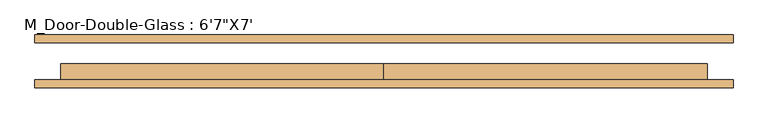
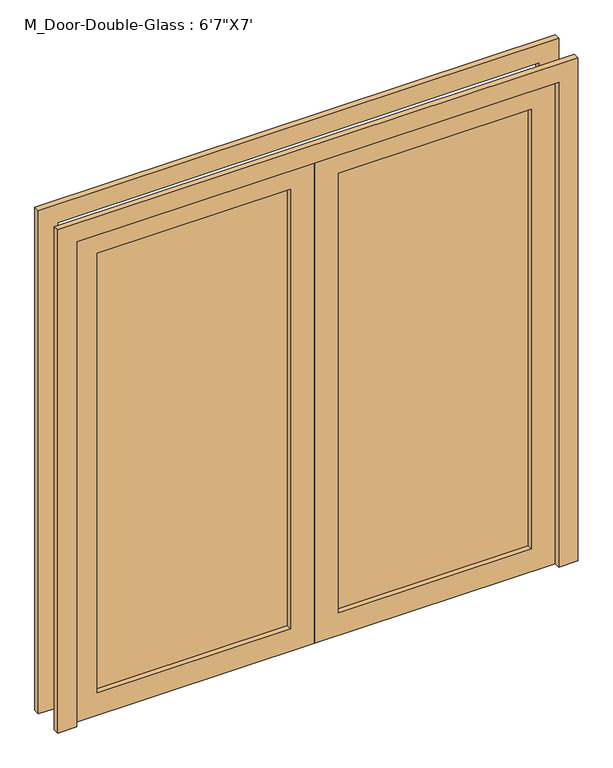
"""IFC4 building model written with IfcOpenShell, lengths in millimetres: door geometry."""

from ifc_helpers import new_model, si_unit, frame, origin, place, context, project, spatial, polyline, outline, extrude, source, transform, mapped, element, save


def door_b125cbd4(model_context):
    return source(origin(), model_context, "Body", "SweptSolid", [
        extrude(outline(polyline([(2133.6, 1003.3), (2133.6, 0.0), (0.0, 0.0), (0.0, 1003.3), (2133.6, 1003.3)]), holes=[polyline([(2033.6, 903.3), (100.0, 903.3), (100.0, 100.0), (2033.6, 100.0), (2033.6, 903.3)])]), frame((0.0, -59.53125, 0.0), z_axis=(0.0, 1.0, 0.0), x_axis=(0.0, 0.0, 1.0)), (0.0, 0.0, 1.0), 50.0),
        extrude(outline(polyline([(2133.6, -1003.3), (0.0, -1003.3), (0.0, 0.0), (2133.6, 0.0), (2133.6, -1003.3)]), holes=[polyline([(2033.6, -903.3), (2033.6, -100.0), (100.0, -100.0), (100.0, -903.3), (2033.6, -903.3)])]), frame((0.0, -59.53125, 0.0), z_axis=(0.0, 1.0, 0.0), x_axis=(0.0, 0.0, 1.0)), (0.0, 0.0, 1.0), 50.0),
        extrude(outline(polyline([(-903.3, -37.70625), (-903.3, -31.35625), (-100.0, -31.35625), (-100.0, -37.70625), (-903.3, -37.70625)])), frame((0.0, 0.0, 100.0), z_axis=(0.0, 0.0, 1.0), x_axis=(1.0, 0.0, 0.0)), (0.0, 0.0, 1.0), 1933.6),
        extrude(outline(polyline([(100.0, -37.70625), (100.0, -31.35625), (903.3, -31.35625), (903.3, -37.70625), (100.0, -37.70625)])), frame((0.0, 0.0, 100.0), z_axis=(0.0, 0.0, 1.0), x_axis=(1.0, 0.0, 0.0)), (0.0, 0.0, 1.0), 1933.6),
        extrude(outline(polyline([(0.0, 1083.3), (2213.6, 1083.3), (2213.6, -1083.3), (0.0, -1083.3), (0.0, -1003.3), (2133.6, -1003.3), (2133.6, 1003.3), (0.0, 1003.3), (0.0, 1083.3)])), frame((0.0, 54.76875, 0.0), z_axis=(0.0, 1.0, 0.0), x_axis=(0.0, 0.0, 1.0)), (0.0, 0.0, 1.0), 25.0),
        extrude(outline(polyline([(0.0, 1083.3), (2213.6, 1083.3), (2213.6, -1083.3), (0.0, -1083.3), (0.0, -1003.3), (2133.6, -1003.3), (2133.6, 1003.3), (0.0, 1003.3), (0.0, 1083.3)])), frame((0.0, -84.53125, 0.0), z_axis=(0.0, 1.0, 0.0), x_axis=(0.0, 0.0, 1.0)), (0.0, 0.0, 1.0), 25.0),
    ])


if __name__ == "__main__":
    model = new_model("IFC4")
    model_context = context("Model", 3, world=origin())
    ifc_project = project(units=[si_unit("LENGTHUNIT", "METRE", prefix="MILLI")], contexts=[model_context])
    site = spatial("IfcSite", under=ifc_project)
    building = spatial("IfcBuilding", under=site)
    placement = place(None, origin())
    door_shape = door_b125cbd4(model_context)
    element("IfcDoor", 1, ObjectType="M_Door-Double-Glass : 6'7\"X7'", at=placement, inside=building, context=model_context, shape_type="MappedRepresentation", body=[
        mapped(door_shape, transform((0.0, 0.0, 0.0), x_axis=(1.0, 0.0, 0.0), y_axis=(0.0, 1.0, 0.0), z_axis=(0.0, 0.0, 1.0))),
    ])
    save(model, "model.ifc")

# Revit data of these elements
# Type "M_Door-Double-Glass : 6'7\"X7'"
#   Type Mark = "16"
#   Construction Type Id = "opn-d45"
#   Assembly Code = "C1020"
#   Analytic Construction = "Wood frame, double glass door "
#   W = 3' - 3 1/2"
#   Thickness = 0' - 1.9685"
#   Thermal Resistance (R) = 1.8150 (h·ft²·°F)/BTU
#   Swing Angle [instance default] = 90.00°
#   Heat Transfer Coefficient (U) = 0.5510 BTU/(h·ft²·°F)
#   Height = 7' - 0"
#   Bottom Rail = 0' - 3.93701"
#   Top Rail = 0' - 3.93701"
#   Stiles = 0' - 3.93701"
#   Trim Projection = 0' - 0.98425"
#   Trim Width = 0' - 3.14961"
#   Width = 6' - 7"
#   Define Thermal Properties by = 1
#   Glazing = Glass
#   Panel Material = Wood - Birch - Solid Stained Light Low Gloss
#   Trim Material = Paint - Sienna
#   Visual Light Transmittance = 0
#   Solar Heat Gain Coefficient = 0
#   Function = (empty or 0)
#   Wall Closure = (empty or 0)
# Element 1 (IfcDoor, "M_Door-Double-Glass : 6'7\"X7'")
#   Materials on its faces: "Wood - Birch - Solid Stained Light Low Gloss", "Paint - Sienna", "Glass"
# Materials
#   "Glass": class "Glass", colour RGB 0 128 192, transparency 0.75, Description = "Soda Lime Glass", Cost = 0
#   "Wood - Birch - Solid Stained Light Low Gloss": class "Wood", colour RGB 210 159 95, transparency 0, Cost = 0
#   "Paint - Sienna": colour RGB 118 70 51, transparency 0, Cost = 0
